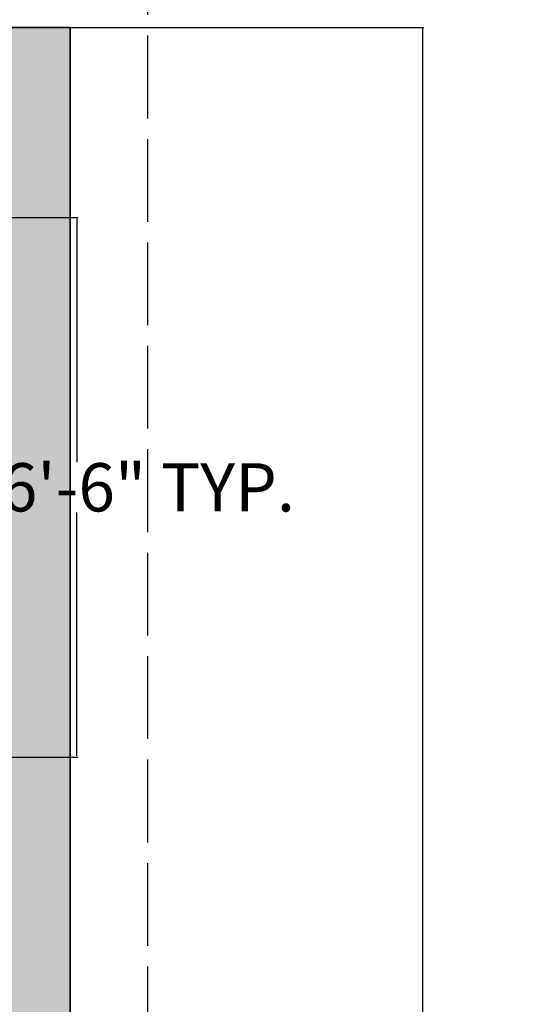
# Model space of a CAD drawing. Units: inches. Extents: x 1316 to 1777, y 813 to 1650.
# Tile 21 of 22: x 1706 to 1777, y 1434 to 1576. Entities that reach past the tile are written whole.
import ezdxf

# ---------------------------------------------------------------- set-up
doc = ezdxf.new("R2010")
doc.units = ezdxf.units.IN
doc.header["$MEASUREMENT"] = 0
doc.linetypes.add('ACAD_ISO02W100', pattern=[15, 12, -3])
for name, color, linetype, lineweight in [('A-ANNO-DIMS', 2, 'Continuous', 18), ('A-WALL-PATT', 250, 'Continuous', 13), ('C-PROP', 8, 'ACAD_ISO02W100', 25), ('walls', 250, 'Continuous', 35)]:
    doc.layers.add(name, color=color, linetype=linetype, lineweight=lineweight)
doc.styles.get("Standard").update_dxf_attribs({"font": 'arial.ttf'})
doc.dimstyles.get("Standard").update_dxf_attribs({"dimtxt": 7, "dimasz": 0.18, "dimexe": 0.18, "dimexo": 0.0625, "dimgap": 0.09, "dimtad": 0, "dimtih": 1, "dimtoh": 1, "dimzin": 0, "dimdsep": 46, "dimlunit": 3, "dimtxsty": 'Standard', "dimcen": 0.09, "dimadec": 0, "dimazin": 0, "dimtfac": 1, "dimtofl": 0, "dimtmove": 0, "dimatfit": 3, "dimfxl": 1, "dimtolj": 1, "dimtzin": 0, "dimarcsym": 0})

# ---------------------------------------------------------------- blocks, each defined once
blk = doc.blocks.new('*D28')
at = {"layer": 'A-ANNO-DIMS', "color": 0, "lineweight": -2, "transparency": 16777216}
for p, q in [((1702.47, 1547.78), (1714.32, 1547.78)), ((1714.14, 1547.6), (1714.14, 1512.32)), ((1714.14, 1469.72), (1714.14, 1504.99)), ((1702.47, 1469.54), (1714.32, 1469.54))]:
    blk.add_line(p, q, dxfattribs=at)
at = {"layer": 'A-ANNO-DIMS', "color": 0, "transparency": 16777216}
for points in [[(1714.11, 1547.6), (1714.17, 1547.6), (1714.14, 1547.78)], [(1714.11, 1469.72), (1714.17, 1469.72), (1714.14, 1469.54)]]:
    blk.add_solid(points, dxfattribs=at)
at = {"layer": 'Defpoints', "color": 0, "transparency": 16777216}
for p in [(1702.41, 1547.78), (1702.41, 1469.54), (1714.14, 1469.54)]:
    blk.add_point(p, dxfattribs=at)
at = {"layer": 'A-ANNO-DIMS', "color": 0, "transparency": 16777216, "insert": (1714.14, 1508.66), "char_height": 7, "attachment_point": 5}
blk.add_mtext('\\A1;BED 6\'-6" TYP.', dxfattribs=at)
blk = doc.blocks.new('*D51')
at = {"layer": 'A-ANNO-DIMS', "color": 0, "lineweight": -2, "transparency": 16777216}
for p, q in [((1713.24, 1575.37), (1764.48, 1575.37)), ((1764.3, 1575.19), (1764.3, 1306.92)), ((1764.3, 1031.35), (1764.3, 1299.62)), ((1713.24, 1031.17), (1764.48, 1031.17))]:
    blk.add_line(p, q, dxfattribs=at)
at = {"layer": 'A-ANNO-DIMS', "color": 0, "transparency": 16777216}
for points in [[(1764.27, 1575.19), (1764.33, 1575.19), (1764.3, 1575.37)], [(1764.27, 1031.35), (1764.33, 1031.35), (1764.3, 1031.17)]]:
    blk.add_solid(points, dxfattribs=at)
at = {"layer": 'Defpoints', "color": 0, "transparency": 16777216}
for p in [(1713.17, 1575.37), (1764.3, 1575.37), (1713.17, 1031.17)]:
    blk.add_point(p, dxfattribs=at)
at = {"layer": 'A-ANNO-DIMS', "color": 0, "transparency": 16777216, "insert": (1764.3, 1303.27), "char_height": 7, "attachment_point": 5}
blk.add_mtext('\\A1;45\'-4"', dxfattribs=at)

msp = doc.modelspace()

# ---------------------------------------------------------------- hatches: boundary and pattern name
at = {"layer": 'A-WALL-PATT'}
h = msp.add_hatch(color=256, dxfattribs=at)
h.dxf.hatch_style = 1
h.paths.add_polyline_path([(1713.173, 1281.369), (1656.173, 1281.369), (1656.173, 1298.258), (1651.673, 1298.258), (1651.673, 1281.369), (1567.673, 1281.369), (1567.673, 1266.995), (1572.173, 1266.995), (1572.173, 1276.869), (1704.173, 1276.869), (1704.173, 1132.869), (1608.64, 1132.869), (1608.64, 1123.869), (1704.173, 1123.869), (1704.173, 1040.173), (1652.869, 1040.173), (1652.869, 1031.173), (1713.173, 1031.173), (1713.173, 1040.173)])
h.paths.add_polyline_path([(1572.173, 1237.955), (1567.673, 1237.955), (1567.673, 1123.869), (1583.146, 1123.869), (1583.146, 1132.869), (1572.173, 1132.869)], flags=17)
h.paths.add_polyline_path([(1510.345, 1566.369), (1524.171, 1566.369), (1524.171, 1571.985), (1524.171, 1575.369), (1445.955, 1575.369), (1445.955, 1566.369), (1505.845, 1566.369), (1505.845, 1469.591), (1510.345, 1469.591), (1510.345, 1471.869), (1529.081, 1471.869), (1529.081, 1476.369), (1510.345, 1476.369)])
h.paths.add_polyline_path([(1609.722, 1575.369), (1545.119, 1575.369), (1545.119, 1566.369), (1570.345, 1566.369), (1570.345, 1476.369), (1562.477, 1476.369), (1562.477, 1471.869), (1570.345, 1471.869), (1570.345, 1469.591), (1574.845, 1469.591), (1574.845, 1566.369), (1609.722, 1566.369)])
h.paths.add_polyline_path([(1713.173, 1575.369), (1655.233, 1575.369), (1655.233, 1566.369), (1704.173, 1566.369), (1704.173, 1434.369), (1574.845, 1434.369), (1574.845, 1440.551), (1574.701, 1440.551), (1570.345, 1440.551), (1570.345, 1429.869), (1597.673, 1429.869), (1597.673, 1408.281), (1602.173, 1408.281), (1602.173, 1429.869), (1704.173, 1429.869), (1704.173, 1410.704), (1707.375, 1410.704), (1713.173, 1410.704)])
h.paths.add_polyline_path([(1713.173, 1383.676), (1704.173, 1383.676), (1704.173, 1369.869), (1602.173, 1369.869), (1602.173, 1379.241), (1597.673, 1379.241), (1597.673, 1365.369), (1713.173, 1365.369)])
h.paths.add_polyline_path([(1444.564, 1429.869), (1510.345, 1429.869), (1510.345, 1440.551), (1505.845, 1440.551), (1505.845, 1434.369), (1386.064, 1434.369), (1386.064, 1566.369), (1400.445, 1566.369), (1400.445, 1575.369), (1377.064, 1575.369), (1377.064, 1412.813), (1380.509, 1412.813), (1386.064, 1412.813), (1386.064, 1429.869), (1440.064, 1429.869), (1440.064, 1401.229), (1444.564, 1401.229)])
h.paths.add_polyline_path([(1444.564, 1372.189), (1440.064, 1372.189), (1440.064, 1369.869), (1386.064, 1369.869), (1386.064, 1378.758), (1377.064, 1378.758), (1377.064, 1349.201), (1381.118, 1349.201), (1386.064, 1349.201), (1386.064, 1365.369), (1440.064, 1365.369), (1440.064, 1322.882), (1444.564, 1322.882)])
h.paths.add_polyline_path([(1510.564, 1295.094), (1506.064, 1295.094), (1506.064, 1245.369), (1386.064, 1245.369), (1386.064, 1272.582), (1377.064, 1272.582), (1377.064, 1212.905), (1380.1, 1212.905), (1386.064, 1212.905), (1386.064, 1240.869), (1510.564, 1240.869)])
h.paths.add_polyline_path([(1386.064, 1163.761), (1377.064, 1163.761), (1377.064, 1063.869), (1419.363, 1063.869), (1419.363, 1072.869), (1386.064, 1072.869)])
h.paths.add_polyline_path([(1510.564, 1072.869), (1469.381, 1072.869), (1469.381, 1063.869), (1501.564, 1063.869), (1501.564, 1033.023), (1501.564, 1031.173), (1540.829, 1031.173), (1540.829, 1036.182, -0.0299535), (1541.068, 1040.173), (1510.564, 1040.173)])
h.paths.add_polyline_path([(1607.369, 1040.173), (1574.225, 1040.173), (1574.225, 1036.182), (1574.225, 1031.173), (1607.369, 1031.173)], flags=17)
h.paths.add_polyline_path([(1637.054, 1040.173), (1624.706, 1040.173), (1624.706, 1031.173), (1637.054, 1031.173)], flags=17)

# ---------------------------------------------------------------- linework, layer by layer
at = {"layer": 'C-PROP'}
msp.add_line((1724.399, 1604.173), (1724.399, 1040.173), dxfattribs=at)
at = {"layer": 'walls'}
for p, q in [((1377.064, 1575.369), (1713.173, 1575.369)), ((1713.173, 1575.369), (1713.173, 1040.173))]:
    msp.add_line(p, q, dxfattribs=at)

# ---------------------------------------------------------------- dimensions: what is measured, and where the dimension line sits
at = {"layer": 'A-ANNO-DIMS'}
dim = msp.add_linear_dim(base=(1764.299, 1575.369), p1=(1713.173, 1031.173), p2=(1713.173, 1575.369), angle=90, dimstyle='Standard', override={"dimdec": 1, "dimlfac": 1, "dimrnd": 0, "dimzin": 1, "dimdsep": 46, "dimlunit": 4, "dimfrac": 2}, dxfattribs=at)
dim.commit()
dim.dimension.update_dxf_attribs({"geometry": '*D51', "text_midpoint": (1764.299, 1303.271)})
dim = msp.add_linear_dim(base=(1714.142, 1469.542), p1=(1702.407, 1547.775), p2=(1702.407, 1469.542), angle=270, text='BED <> TYP.', dimstyle='Standard', override={"dimdec": 1, "dimlfac": 1, "dimrnd": 0, "dimzin": 1, "dimdsep": 46, "dimlunit": 4, "dimfrac": 2}, dxfattribs=at)
dim.commit()
dim.dimension.update_dxf_attribs({"geometry": '*D28', "text_midpoint": (1714.142, 1508.658)})

doc.saveas('drawing.dxf')
